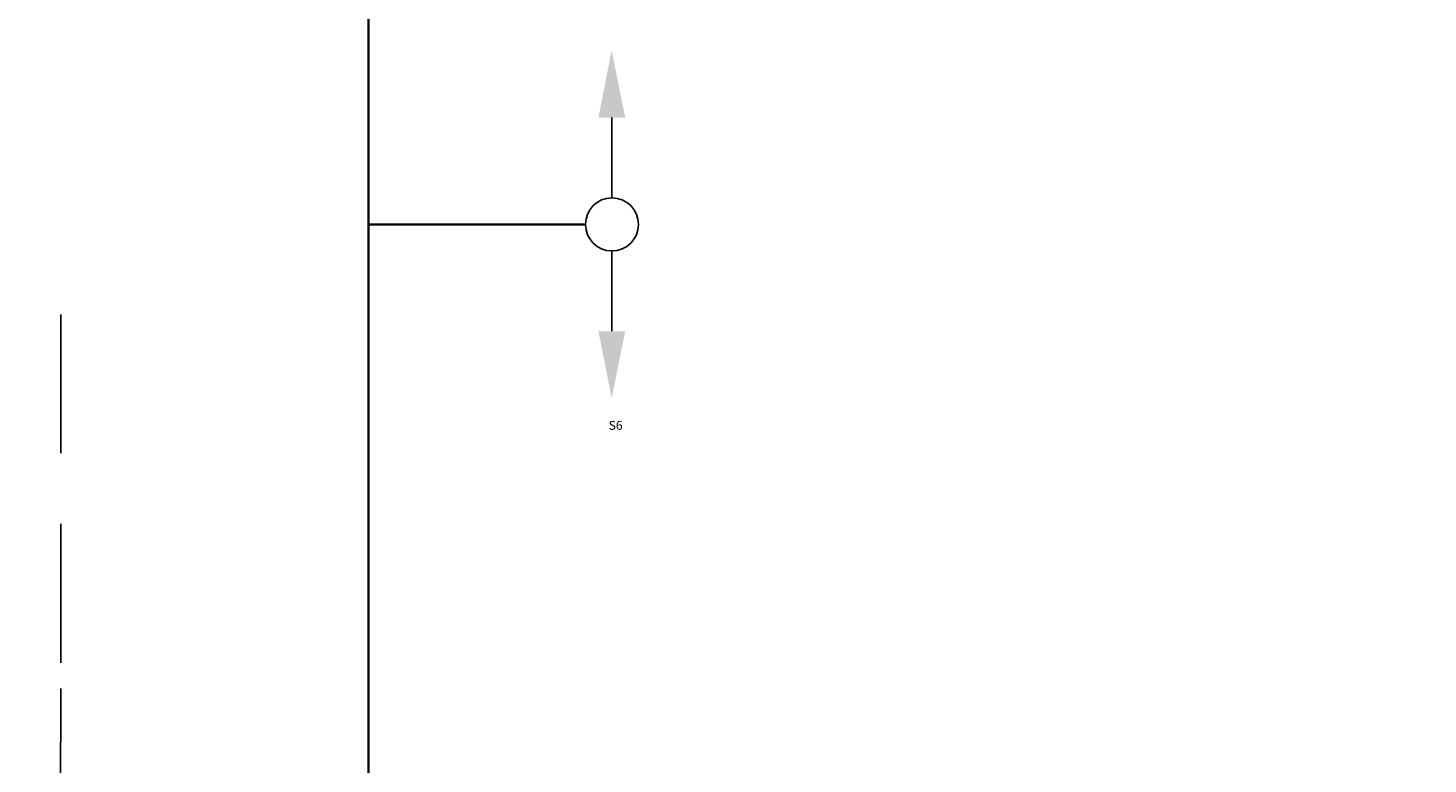
# Model space of a CAD drawing. Units: millimetres. Extents: x 353872 to 441597, y 126154 to 187356.
# Tile 13 of 28: x 392355 to 395281, y 152234 to 153772. Entities that reach past the tile are written whole.
import ezdxf

# ---------------------------------------------------------------- set-up
doc = ezdxf.new("R2010")
doc.units = ezdxf.units.MM
doc.layers.add('AC-UINT', color=2, linetype='Continuous')
for name, color, linetype, lineweight in [('P-ANNO-TEXT', 7, 'Continuous', 25), ('P-INST', 6, 'Continuous', 25), ('P-PIPE', 3, 'Continuous', 35), ('P-PIPE-FITT', 6, 'Continuous', 25)]:
    doc.layers.add(name, color=color, linetype=linetype, lineweight=lineweight)
doc.styles.get("Standard").update_dxf_attribs({"font": 'arial.ttf'})

# ---------------------------------------------------------------- blocks, each defined once
blk = doc.blocks.new('DFSG')
at = {"layer": 'AC-UINT', "ltscale": 3}
blk.add_line((94.3237, -27.1601), (94.091, -27.1601), dxfattribs=at)
blk.add_solid([(94.091, -27.1214), (94.0909, -27.1989), (93.8965, -27.1598)], dxfattribs=at)

msp = doc.modelspace()

# ---------------------------------------------------------------- linework, layer by layer
at = {"layer": 'P-INST'}
for p, q in [((392423.75, 153173.15), (392423.75, 152883.12)), ((392423.75, 152735.08), (392423.75, 152445.05))]:
    msp.add_line(p, q, dxfattribs=at)
msp.add_circle((393575.41, 153361.16), 55.35, dxfattribs=at)
at = {"layer": 'P-PIPE'}
msp.add_line((393066.71, 153361.16), (393520.06, 153361.16), dxfattribs=at)
msp.add_lwpolyline([(393066.71, 149319.73), (393066.71, 175399.89), (426420.76, 175399.89)], dxfattribs=at)

# ---------------------------------------------------------------- block references
at = {"layer": 'P-PIPE-FITT'}
for p, xscale, yscale, zscale, rotation in [((373891.93, 221407.87), -721.1287546377986, 721.1287546377986, 721.1287546377986, 90.08218228964184), ((373891.93, 85314.44), 721.1287546377986, 721.1287546377986, 721.1287546377986, 89.91781771035816), ((344986.64, -11465.79), 1737.899325704125, 1737.899325704125, 1737.899325704125, 89.91781771039466)]:
    msp.add_blockref('DFSG', p, dxfattribs=dict(at, xscale=xscale, yscale=yscale, zscale=zscale, rotation=rotation))

# ---------------------------------------------------------------- texts
at = {"layer": 'P-ANNO-TEXT'}
msp.add_text('S6', height=18.55, dxfattribs=at).set_placement((393568.56, 152931.92))

doc.saveas('drawing.dxf')
